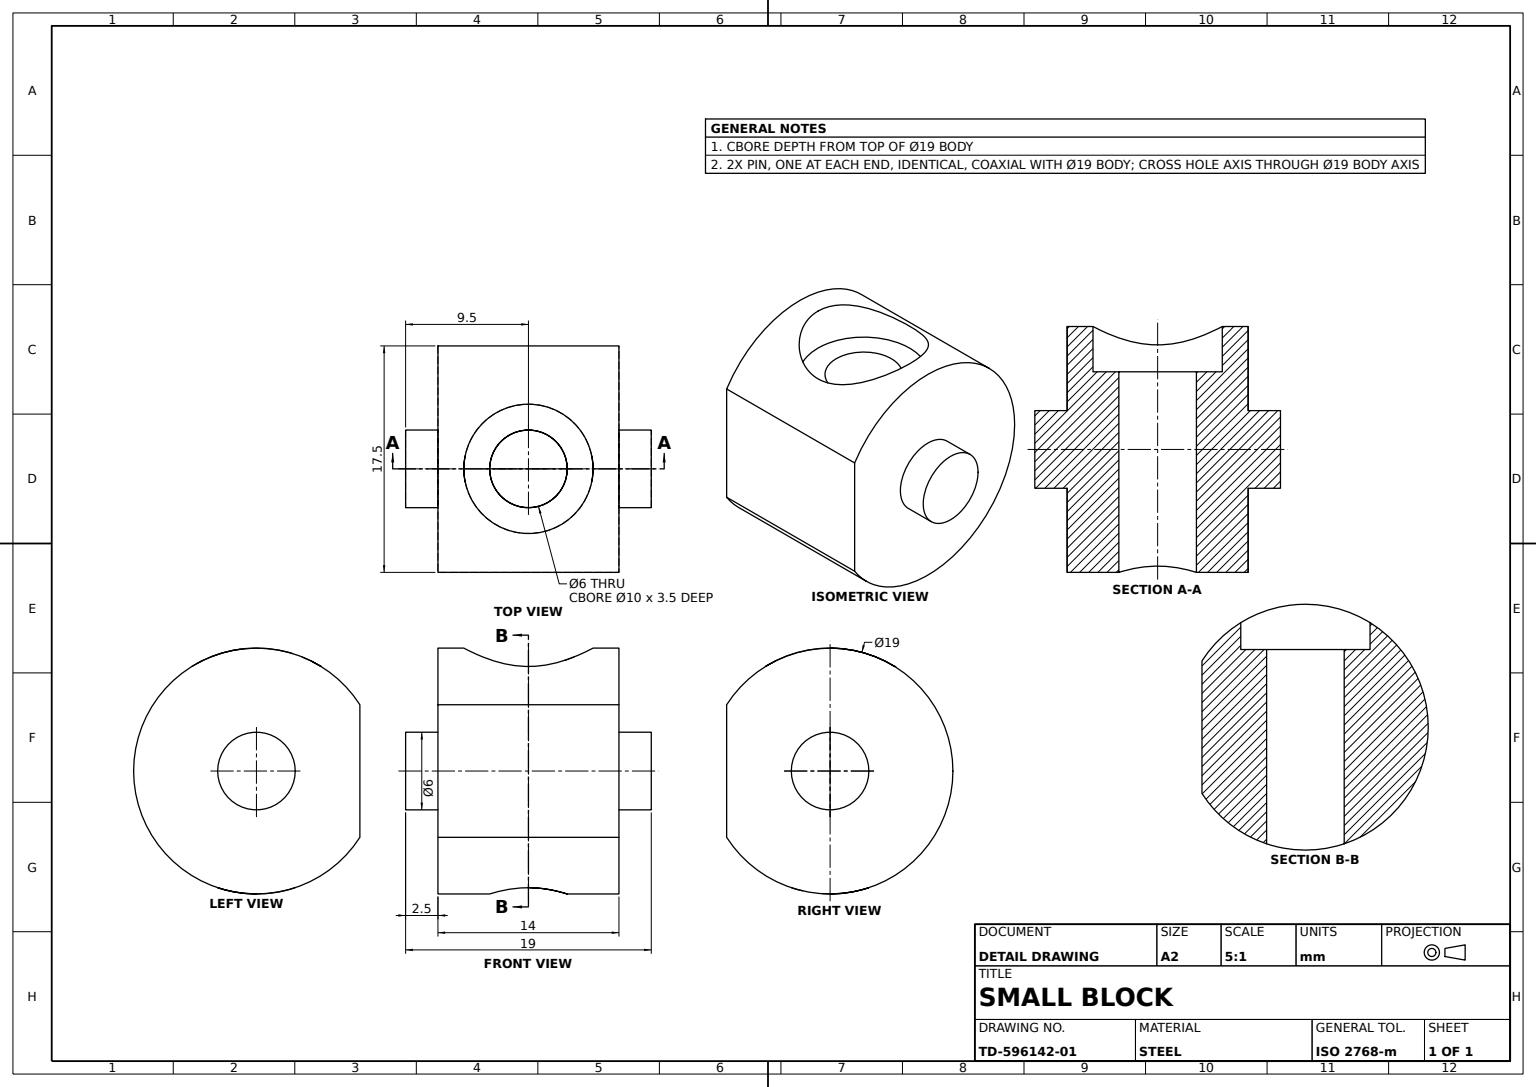
from build123d import *

# Parameters (mm, degrees)
BUSHING_BODY_DEPTH          = 14
FRONT_PIVOT_PIN_PROFILE_6_R = 3
FRONT_PIVOT_PIN_6_DEPTH     = 2.5
REAR_START                  = 2.5
REAR_PIVOT_PIN_PROFILE_6_R  = 3
REAR_PIVOT_PIN_6_DEPTH      = 2.5
CROSS_COUNTERBORE_PROFILE_R = 5
CROSS_COUNTERBORE_DEPTH     = 4
CROSS_HOLE_PROFILE_6_R      = 3
CROSS_HOLE_6_DEPTH          = 16


with BuildPart() as part:
    # Body Profile Ø19 D-Flat → Bushing Body (new body)
    with BuildSketch(Plane.XY):
        with BuildLine():
            Line((8, 5.123475383), (8, -5.123475383))
            ThreePointArc((8, -5.123475383), (-9.5, 0), (8, 5.123475383))
        make_face()
    extrude(amount=BUSHING_BODY_DEPTH)

    # Front Pivot Pin Profile Ø6 → Front Pivot Pin Ø6 (add)
    with BuildSketch(Plane.XY.offset(14)):
        Circle(FRONT_PIVOT_PIN_PROFILE_6_R)
    extrude(amount=FRONT_PIVOT_PIN_6_DEPTH)

    # Rear Pivot Pin Profile Ø6 → Rear Pivot Pin Ø6 (add)
    with BuildSketch(Plane(origin=(0, 0, 0), x_dir=(-1, 0, 0), z_dir=(0, 0, -1)).offset(REAR_START)):
        with Locations(Location((0, 0, 0), (0, 0, 180))):
            Circle(REAR_PIVOT_PIN_PROFILE_6_R)
    extrude(amount=-REAR_PIVOT_PIN_6_DEPTH)

    # Cross Counterbore Profile → Cross Counterbore (cut)
    with BuildSketch(Plane(origin=(0, 10, 0), x_dir=(1, 0, 0), z_dir=(0, 1, 0))):
        with Locations(Location((0, -7, 0), (0, 0, 270))):
            Circle(CROSS_COUNTERBORE_PROFILE_R)
    extrude(amount=-CROSS_COUNTERBORE_DEPTH, mode=Mode.SUBTRACT)

    # Cross Hole Profile Ø6 → Cross Hole Ø6 (cut)
    with BuildSketch(Plane(origin=(0, 6, 0), x_dir=(1, 0, 0), z_dir=(0, 1, 0))):
        with Locations(Location((0, -7, 0), (0, 0, 270))):
            Circle(CROSS_HOLE_PROFILE_6_R)
    extrude(amount=-CROSS_HOLE_6_DEPTH, mode=Mode.SUBTRACT)


solid = part.part
